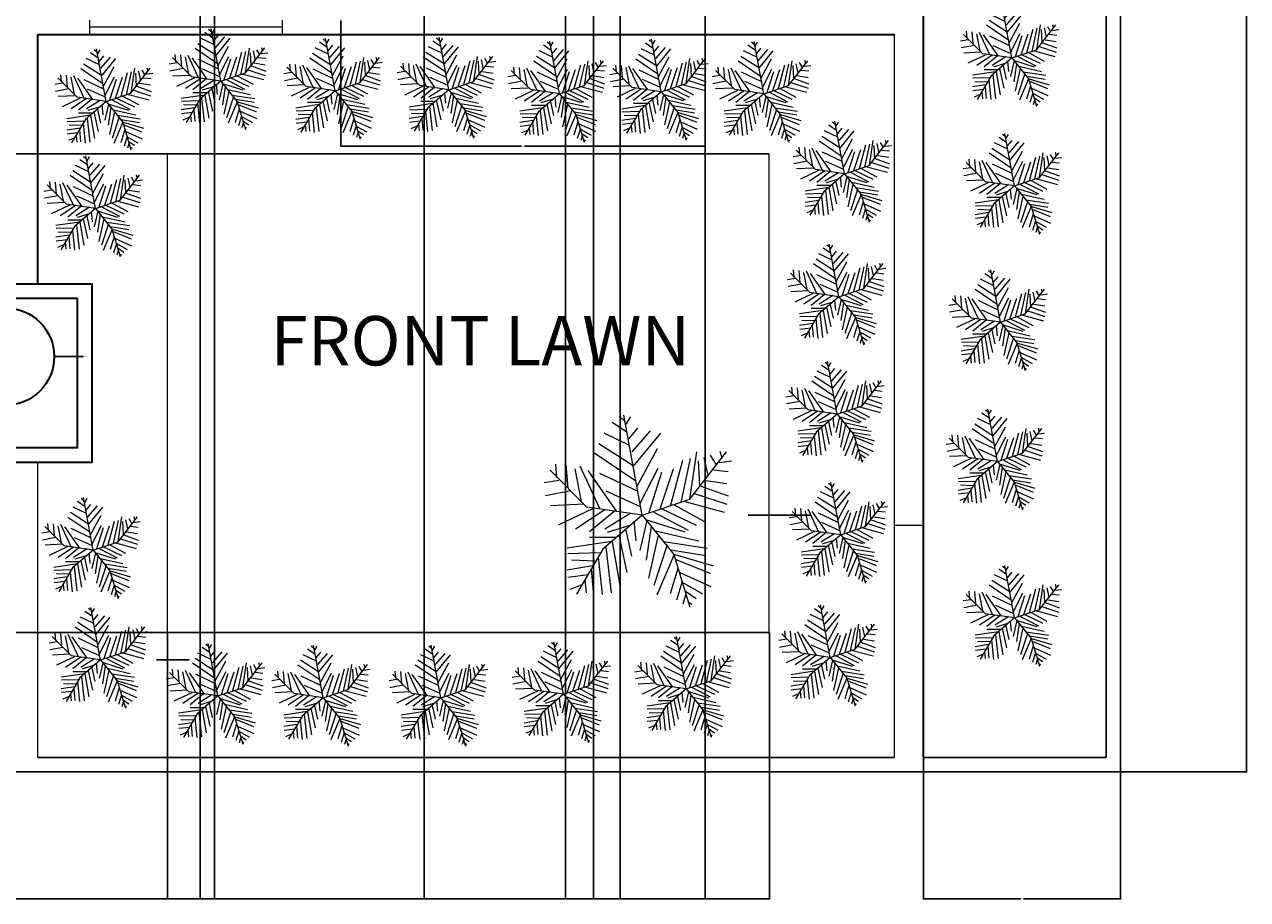
# Model space of a CAD drawing. Units: inches. Extents: x -86 to 773, y -188 to 560.
# Tile 4 of 6: x 392 to 773, y -188 to 85. Entities that reach past the tile are written whole.
import ezdxf

# ---------------------------------------------------------------- set-up
doc = ezdxf.new("R2010")
doc.units = ezdxf.units.IN
doc.header["$MEASUREMENT"] = 0
for name, color, linetype, lineweight in [('A-ANNO-DIMS', 2, 'Continuous', 18), ('A-AREA-IDEN', 7, 'Continuous', 25), ('A-COLS', 7, 'Continuous', 35), ('A-GLAZ', 7, 'Continuous', 18), ('A-WALL', 7, 'Continuous', 35), ('C-PROP', 7, 'Continuous', 25), ('L-HRDS', 7, 'Continuous', 18), ('L-PLNT', 8, 'Continuous', 13), ('L-PLNT-TREE', 8, 'Continuous', 9)]:
    doc.layers.add(name, color=color, linetype=linetype, lineweight=lineweight)
doc.styles.get("Standard").update_dxf_attribs({"font": 'arial.ttf'})
doc.dimstyles.get("Standard").update_dxf_attribs({"dimtxt": 0.18, "dimasz": 0.18, "dimexe": 0.18, "dimexo": 0.0625, "dimgap": 0.09, "dimtad": 0, "dimtih": 1, "dimtoh": 1, "dimdec": 4, "dimzin": 0, "dimdsep": 46, "dimtxsty": 'Standard', "dimcen": 0.09, "dimadec": 0, "dimazin": 0, "dimtfac": 1, "dimtdec": 4, "dimtofl": 0, "dimtmove": 0, "dimatfit": 3, "dimfxl": 1, "dimtolj": 1, "dimtzin": 0, "dimarcsym": 0})

# ---------------------------------------------------------------- blocks, each defined once
blk = doc.blocks.new('Trees - Metric')
for p, q in [((-258.7244, 1362.456), (-332.3336, 1421.4348)), ((0, 0), (-266.7, 1447.8)), ((-231.1146, 1315.2628), (-166.7002, 1421.4348)), ((-221.9198, 1197.3052), (-433.5526, 1338.8594)), ((-194.31, 1102.9442), (-65.4812, 1256.284)), ((-185.1152, 1008.5578), (-553.1612, 1185.4942)), ((-148.3106, 914.1968), (118.5418, 1220.9018)), ((-129.8956, 701.8528), (265.7602, 1185.4942)), ((-93.091, 489.5342), (-700.3796, 902.3858)), ((-129.8956, 713.6638), (-626.7704, 1032.1544)), ((-74.7014, 418.7444), (219.7608, 961.39)), ((685.8, 228.6), (1219.2, 914.4)), ((689.0258, 230.0224), (790.2448, 914.1968)), ((1121.4862, 925.9824), (1149.0706, 831.6214)), ((-1234.059, 536.7274), (-1252.4486, 737.2604)), ((-1105.2302, 725.4494), (-1077.6458, 395.1732)), ((-902.8176, 713.6638), (-617.5756, 100.2538)), ((412.9786, 147.447), (587.8068, 796.2392)), ((560.197, 182.8292), (698.2206, 819.8358)), ((808.6344, 784.4282), (827.0494, 418.7444)), ((891.4384, 831.6214), (946.658, 572.1096)), ((983.4626, 867.0036), (1066.2666, 725.4494)), ((1112.2914, 760.8316), (1296.3144, 784.4282)), ((-800.1, 114.3), (-1333.5, 647.7)), ((-976.4268, 666.4706), (-884.4026, 194.6402)), ((-369.1382, 53.086), (-783.1836, 642.874)), ((-617.5756, 607.4918), (-74.7014, 347.98)), ((-28.6766, 171.0436), (228.9556, 678.2816)), ((100.1268, 41.275), (284.1498, 619.2774)), ((256.5654, 88.4682), (449.7832, 666.4706)), ((1029.462, 654.685), (1241.0948, 631.0884)), ((-1206.4492, 501.3198), (-1418.082, 465.9376)), ((845.439, 418.7444), (1241.0948, 277.1902)), ((919.0482, 501.3198), (1222.6798, 454.152)), ((-1031.621, 347.98), (-1399.667, 277.1902)), ((-525.5514, 347.98), (-28.6766, 123.8504)), ((0, 0), (685.8, 228.6)), ((615.4166, 194.6402), (1185.8752, 41.275)), ((753.4148, 312.5978), (1222.6798, 159.2326)), ((-847.598, 159.2326), (-1326.0578, 135.636)), ((-718.7946, 88.4682), (-1215.644, -147.447)), ((-543.9664, 76.6572), (-967.2066, -206.4512)), ((0, 0), (-800.1, 114.3)), ((-405.9428, 53.086), (-764.794, -241.8334)), ((0, 0), (-571.5, -495.3)), ((-166.7002, 29.4894), (-543.9664, -206.4512)), ((0, 0), (457.2, -571.5)), ((164.5412, 41.275), (661.416, -218.2368)), ((284.1498, 88.4682), (781.0246, -147.447)), ((458.978, 147.447), (891.4384, -88.4682)), ((-166.7002, -147.447), (-507.1618, -253.619)), ((-120.7008, -88.4682), (-93.091, -371.5766)), ((63.3222, -76.6826), (-37.8714, -513.1308)), ((44.9326, -64.897), (615.4166, -241.8334)), ((127.7366, -159.258), (54.1274, -654.685)), ((-387.5278, -324.4088), (-764.794, -324.4088)), ((-341.5284, -289.0012), (-221.9198, -831.6214)), ((-240.3094, -218.2368), (-157.5054, -595.7062)), ((228.9556, -289.0012), (90.932, -914.1968)), ((192.151, -230.0224), (817.8292, -371.5766)), ((-442.7474, -383.3876), (-1086.8406, -477.7486)), ((-571.5, -495.3), (-952.5, -1143)), ((-525.5514, -465.963), (-451.9422, -1126.5408)), ((-433.5526, -383.3876), (-323.1134, -1020.3688)), ((357.759, -430.5554), (164.5412, -1020.3688)), ((311.7596, -383.3876), (937.4378, -477.7486)), ((412.9786, -501.3452), (919.0482, -583.9206)), ((-617.5756, -548.5384), (-1077.6458, -560.324)), ((-681.9646, -666.496), (-1022.4262, -654.685)), ((-635.9652, -607.5172), (-580.771, -1150.1374)), ((458.978, -572.1096), (210.5406, -1161.923)), ((457.2, -571.5), (685.8, -1333.5)), ((468.1982, -572.1096), (1029.462, -737.2604)), ((486.5878, -642.8994), (983.4626, -843.4324)), ((-718.7946, -737.2604), (-1086.8406, -796.2392)), ((-783.1836, -867.029), (-1077.6458, -902.4112)), ((-737.1842, -784.4536), (-709.5744, -1114.7298)), ((514.1976, -772.6426), (403.7838, -1138.3264)), ((541.8074, -831.6214), (992.6574, -1032.1544)), ((-875.2078, -1008.5832), (-1040.8412, -1079.3476)), ((-829.2084, -937.7934), (-810.7934, -1126.5408)), ((578.612, -961.39), (495.7826, -1232.7128)), ((578.612, -973.1756), (873.0488, -1138.3264)), ((624.6114, -1161.923), (587.8068, -1291.6916)), ((624.6114, -1102.9442), (781.0246, -1209.1162)), ((679.8056, -1268.095), (716.6102, -1291.6916))]:
    blk.add_line(p, q)
blk = doc.blocks.new('WIN-60-W4_5')
for p, q in [((0, 4.5), (0, 0)), ((60, 4.5), (60, 0)), ((60, 2.25), (0, 2.25))]:
    blk.add_line(p, q)
blk = doc.blocks.new('PORCH-COLUMN-PLINTH')
for points in [[(0, 55.74), (51.99, 55.74), (51.99, 0), (0, 0)], [(4.5, 51.24), (47.49, 51.24), (47.49, 4.5), (4.5, 4.5)]]:
    blk.add_lwpolyline(points, close=True)
blk = doc.blocks.new('*D46')
at = {"layer": 'A-ANNO-DIMS', "color": 0, "lineweight": -2, "transparency": 16777216}
for p, q in [((733.51, 486.66), (772.88, 486.66)), ((772.7, 486.48), (772.7, 169.55)), ((772.7, -147.74), (772.7, 169.19)), ((733.51, -147.92), (772.88, -147.92))]:
    blk.add_line(p, q, dxfattribs=at)
at = {"layer": 'A-ANNO-DIMS', "color": 0, "transparency": 16777216}
for points in [[(772.67, 486.48), (772.73, 486.48), (772.7, 486.66)], [(772.67, -147.74), (772.73, -147.74), (772.7, -147.92)]]:
    blk.add_solid(points, dxfattribs=at)
at = {"layer": 'Defpoints', "color": 0, "transparency": 16777216}
for p in [(733.45, 486.66), (772.7, 486.66), (733.45, -147.92)]:
    blk.add_point(p, dxfattribs=at)
at = {"layer": 'A-ANNO-DIMS', "color": 0, "transparency": 16777216, "insert": (772.7, 169.37), "char_height": 0.18, "attachment_point": 5}
blk.add_mtext('\\A1;634.6', dxfattribs=at)
blk = doc.blocks.new('*D48')
at = {"layer": 'A-ANNO-DIMS', "color": 0, "lineweight": -2, "transparency": 16777216}
for p, q in [((672.01, -143.48), (672.01, -187.76)), ((733.45, -147.98), (733.45, -187.76)), ((672.19, -187.58), (702.34, -187.58)), ((733.27, -187.58), (703.13, -187.58))]:
    blk.add_line(p, q, dxfattribs=at)
at = {"layer": 'A-ANNO-DIMS', "color": 0, "transparency": 16777216}
for points in [[(672.19, -187.55), (672.19, -187.61), (672.01, -187.58)], [(733.27, -187.55), (733.27, -187.61), (733.45, -187.58)]]:
    blk.add_solid(points, dxfattribs=at)
at = {"layer": 'Defpoints', "color": 0, "transparency": 16777216}
for p in [(672.01, -143.42), (733.45, -147.92), (733.45, -187.58)]:
    blk.add_point(p, dxfattribs=at)
at = {"layer": 'A-ANNO-DIMS', "color": 0, "transparency": 16777216, "insert": (702.73, -187.58), "char_height": 0.18, "attachment_point": 5}
blk.add_mtext('\\A1;61.44', dxfattribs=at)
blk = doc.blocks.new('*D52')
at = {"layer": 'A-ANNO-DIMS', "color": 0, "lineweight": -2, "transparency": 16777216}
for p, q in [((436.42, -104.53), (436.42, -187.76)), ((623.99, -104.5), (623.99, -187.76)), ((436.6, -187.58), (529.75, -187.58)), ((623.81, -187.58), (530.66, -187.58))]:
    blk.add_line(p, q, dxfattribs=at)
at = {"layer": 'A-ANNO-DIMS', "color": 0, "transparency": 16777216}
for points in [[(436.6, -187.55), (436.6, -187.61), (436.42, -187.58)], [(623.81, -187.55), (623.81, -187.61), (623.99, -187.58)]]:
    blk.add_solid(points, dxfattribs=at)
at = {"layer": 'Defpoints', "color": 0, "transparency": 16777216}
for p in [(436.42, -104.46), (623.99, -104.44), (623.99, -187.58)]:
    blk.add_point(p, dxfattribs=at)
at = {"layer": 'A-ANNO-DIMS', "color": 0, "transparency": 16777216, "insert": (530.2, -187.58), "char_height": 0.18, "attachment_point": 5}
blk.add_mtext('\\A1;187.57', dxfattribs=at)
blk = doc.blocks.new('*D53')
at = {"layer": 'A-ANNO-DIMS', "color": 0, "lineweight": -2, "transparency": 16777216}
for p, q in [((623.74, 44.83), (-85.98, 44.83)), ((-85.8, 44.65), (-85.8, -29.62)), ((-85.8, -104.26), (-85.8, -29.99)), ((623.93, -104.44), (-85.98, -104.44))]:
    blk.add_line(p, q, dxfattribs=at)
at = {"layer": 'A-ANNO-DIMS', "color": 0, "transparency": 16777216}
for points in [[(-85.83, 44.65), (-85.77, 44.65), (-85.8, 44.83)], [(-85.83, -104.26), (-85.77, -104.26), (-85.8, -104.44)]]:
    blk.add_solid(points, dxfattribs=at)
at = {"layer": 'Defpoints', "color": 0, "transparency": 16777216}
for p in [(623.81, 44.83), (-85.8, -104.44), (623.99, -104.44)]:
    blk.add_point(p, dxfattribs=at)
at = {"layer": 'A-ANNO-DIMS', "color": 0, "transparency": 16777216, "insert": (-85.8, -29.81), "char_height": 0.18, "attachment_point": 5}
blk.add_mtext('\\A1;149.27', dxfattribs=at)
blk = doc.blocks.new('*D54')
at = {"layer": 'A-ANNO-DIMS', "color": 0, "lineweight": -2, "transparency": 16777216}
for p, q in [((451.03, 440.67), (451.03, -187.76)), ((569.11, 440.67), (569.11, -187.76)), ((451.21, -187.58), (509.62, -187.58)), ((568.93, -187.58), (510.53, -187.58))]:
    blk.add_line(p, q, dxfattribs=at)
at = {"layer": 'A-ANNO-DIMS', "color": 0, "transparency": 16777216}
for points in [[(451.21, -187.55), (451.21, -187.61), (451.03, -187.58)], [(568.93, -187.55), (568.93, -187.61), (569.11, -187.58)]]:
    blk.add_solid(points, dxfattribs=at)
at = {"layer": 'Defpoints', "color": 0, "transparency": 16777216}
for p in [(451.03, 440.74), (569.11, 440.74), (569.11, -187.58)]:
    blk.add_point(p, dxfattribs=at)
at = {"layer": 'A-ANNO-DIMS', "color": 0, "transparency": 16777216, "insert": (510.07, -187.58), "char_height": 0.18, "attachment_point": 5}
blk.add_mtext('\\A1;118.08', dxfattribs=at)
blk = doc.blocks.new('*D65')
at = {"layer": 'A-ANNO-DIMS', "color": 0, "lineweight": -2, "transparency": 16777216}
for p, q in [((446.53, 366.45), (446.53, -187.76)), ((215.06, 361.95), (215.06, -187.76)), ((215.24, -187.58), (330.33, -187.58)), ((446.35, -187.58), (331.26, -187.58))]:
    blk.add_line(p, q, dxfattribs=at)
at = {"layer": 'A-ANNO-DIMS', "color": 0, "transparency": 16777216}
for points in [[(215.24, -187.55), (215.24, -187.61), (215.06, -187.58)], [(446.35, -187.55), (446.35, -187.61), (446.53, -187.58)]]:
    blk.add_solid(points, dxfattribs=at)
at = {"layer": 'Defpoints', "color": 0, "transparency": 16777216}
for p in [(446.53, 366.52), (215.06, 362.02), (446.53, -187.58)]:
    blk.add_point(p, dxfattribs=at)
at = {"layer": 'A-ANNO-DIMS', "color": 0, "transparency": 16777216, "insert": (330.8, -187.58), "char_height": 0.18, "attachment_point": 5}
blk.add_mtext('\\A1;231.47', dxfattribs=at)
blk = doc.blocks.new('*D71')
at = {"layer": 'A-ANNO-DIMS', "color": 0, "lineweight": -2, "transparency": 16777216}
for p, q in [((490.39, 86.43), (490.39, 47.07)), ((603.97, 86.43), (603.97, 47.07)), ((490.57, 47.25), (546.73, 47.25)), ((603.79, 47.25), (547.64, 47.25))]:
    blk.add_line(p, q, dxfattribs=at)
at = {"layer": 'A-ANNO-DIMS', "color": 0, "transparency": 16777216}
for points in [[(490.57, 47.28), (490.57, 47.22), (490.39, 47.25)], [(603.79, 47.28), (603.79, 47.22), (603.97, 47.25)]]:
    blk.add_solid(points, dxfattribs=at)
at = {"layer": 'Defpoints', "color": 0, "transparency": 16777216}
for p in [(490.39, 86.5), (603.97, 86.5), (490.39, 47.25)]:
    blk.add_point(p, dxfattribs=at)
at = {"layer": 'A-ANNO-DIMS', "color": 0, "transparency": 16777216, "insert": (547.18, 47.25), "char_height": 0.18, "attachment_point": 5}
blk.add_mtext('\\A1;113.58', dxfattribs=at)
blk = doc.blocks.new('*D72')
at = {"layer": 'A-ANNO-DIMS', "color": 0, "lineweight": -2, "transparency": 16777216}
for p, q in [((560.48, 361.95), (560.48, -187.76)), ((603.97, 361.95), (603.97, -187.76)), ((560.66, -187.58), (581.76, -187.58)), ((603.79, -187.58), (582.69, -187.58))]:
    blk.add_line(p, q, dxfattribs=at)
at = {"layer": 'A-ANNO-DIMS', "color": 0, "transparency": 16777216}
for points in [[(560.66, -187.55), (560.66, -187.61), (560.48, -187.58)], [(603.79, -187.55), (603.79, -187.61), (603.97, -187.58)]]:
    blk.add_solid(points, dxfattribs=at)
at = {"layer": 'Defpoints', "color": 0, "transparency": 16777216}
for p in [(560.48, 362.01), (603.97, 362.02), (603.97, -187.58)]:
    blk.add_point(p, dxfattribs=at)
at = {"layer": 'A-ANNO-DIMS', "color": 0, "transparency": 16777216, "insert": (582.22, -187.58), "char_height": 0.18, "attachment_point": 5}
blk.add_mtext('\\A1;43.496', dxfattribs=at)
blk = doc.blocks.new('*D74')
at = {"layer": 'A-ANNO-DIMS', "color": 0, "lineweight": -2, "transparency": 16777216}
for p, q in [((516.4, 181.21), (516.4, -187.76)), ((577.46, 181.21), (577.46, -187.76)), ((516.58, -187.58), (546.54, -187.58)), ((577.28, -187.58), (547.32, -187.58))]:
    blk.add_line(p, q, dxfattribs=at)
at = {"layer": 'A-ANNO-DIMS', "color": 0, "transparency": 16777216}
for points in [[(516.58, -187.55), (516.58, -187.61), (516.4, -187.58)], [(577.28, -187.55), (577.28, -187.61), (577.46, -187.58)]]:
    blk.add_solid(points, dxfattribs=at)
at = {"layer": 'Defpoints', "color": 0, "transparency": 16777216}
for p in [(516.4, 181.27), (577.46, 181.27), (577.46, -187.58)]:
    blk.add_point(p, dxfattribs=at)
at = {"layer": 'A-ANNO-DIMS', "color": 0, "transparency": 16777216, "insert": (546.93, -187.58), "char_height": 0.18, "attachment_point": 5}
blk.add_mtext('\\A1;61.06', dxfattribs=at)
blk = doc.blocks.new('*D89')
at = {"layer": 'A-ANNO-DIMS', "color": 0, "lineweight": -2, "transparency": 16777216}
for p, q in [((584.28, -67.83), (584.46, -67.83)), ((584.37, -67.92), (584.37, -67.74)), ((636.91, -67.83), (617.39, -67.83))]:
    blk.add_line(p, q, dxfattribs=at)
at = {"layer": 'A-ANNO-DIMS', "color": 0, "transparency": 16777216}
blk.add_solid([(617.39, -67.8), (617.39, -67.86), (617.21, -67.83)], dxfattribs=at)
at = {"layer": 'Defpoints', "color": 0, "transparency": 16777216}
for p in [(551.53, -67.83), (617.21, -67.83)]:
    blk.add_point(p, dxfattribs=at)
at = {"layer": 'A-ANNO-DIMS', "color": 0, "transparency": 16777216, "insert": (637.41, -67.83), "char_height": 0.18, "attachment_point": 5}
blk.add_mtext('\\A1;∅65.68', dxfattribs=at)
blk = doc.blocks.new('*D90')
at = {"layer": 'A-ANNO-DIMS', "color": 0, "lineweight": -2, "transparency": 16777216}
for p, q in [((415.45, -113.03), (415.63, -113.03)), ((415.54, -113.12), (415.54, -112.94)), ((443.09, -113.03), (432.94, -113.03))]:
    blk.add_line(p, q, dxfattribs=at)
at = {"layer": 'A-ANNO-DIMS', "color": 0, "transparency": 16777216}
blk.add_solid([(432.94, -113), (432.94, -113.06), (432.76, -113.03)], dxfattribs=at)
at = {"layer": 'Defpoints', "color": 0, "transparency": 16777216}
for p in [(398.32, -113.03), (432.76, -113.03)]:
    blk.add_point(p, dxfattribs=at)
at = {"layer": 'A-ANNO-DIMS', "color": 0, "transparency": 16777216, "insert": (443.84, -113.03), "char_height": 0.18, "attachment_point": 5}
blk.add_mtext('\\A1;47X ∅34.44', dxfattribs=at)
blk = doc.blocks.new('*D92')
at = {"layer": 'A-ANNO-DIMS', "color": 0, "lineweight": -2, "transparency": 16777216}
for p, q in [((385.79, -18.42), (385.97, -18.42)), ((385.88, -18.51), (385.88, -18.33)), ((410.18, -18.42), (401.25, -18.42))]:
    blk.add_line(p, q, dxfattribs=at)
at = {"layer": 'A-ANNO-DIMS', "color": 0, "transparency": 16777216}
blk.add_solid([(401.25, -18.39), (401.25, -18.45), (401.07, -18.42)], dxfattribs=at)
at = {"layer": 'Defpoints', "color": 0, "transparency": 16777216}
for p in [(370.7, -18.42), (401.07, -18.42)]:
    blk.add_point(p, dxfattribs=at)
at = {"layer": 'A-ANNO-DIMS', "color": 0, "transparency": 16777216, "insert": (410.67, -18.42), "char_height": 0.18, "attachment_point": 5}
blk.add_mtext('\\A1;∅30.37', dxfattribs=at)

msp = doc.modelspace()

# ---------------------------------------------------------------- linework, layer by layer
at = {"layer": 'A-COLS'}
msp.add_circle((385.883, -18.4243), 15.1853, dxfattribs=at)
at = {"layer": 'A-WALL'}
for p, q in [((672.0115, -143.4172), (672.0115, 366.5167)), ((395.9662, 4.3272), (395.9662, 81.9967))]:
    msp.add_line(p, q, dxfattribs=at)
msp.add_lwpolyline([(395.9662, 81.9967), (663.0115, 81.9967)], dxfattribs=at)
at = {"layer": 'C-PROP'}
for p, q in [((733.4515, -147.9172), (733.4515, 486.6589)), ((728.9515, -143.4172), (728.9515, 482.1589)), ((395.9662, -143.4172), (663.0115, -143.4172)), ((672.0115, -143.4172), (728.9515, -143.4172)), ((269.2915, -147.9172), (733.4515, -147.9172))]:
    msp.add_line(p, q, dxfattribs=at)
at = {"layer": 'L-HRDS'}
for p, q in [((663.0115, -143.4172), (663.0115, 81.9967)), ((395.9662, -143.4172), (395.9662, -51.4118))]:
    msp.add_line(p, q, dxfattribs=at)
msp.add_lwpolyline([(663.0115, -70.9433), (672.0115, -70.9433)], dxfattribs=at)
at = {"layer": 'L-PLNT'}
msp.add_lwpolyline([(436.4196, 44.8288), (623.8051, 44.8288), (623.8051, -104.464), (436.4196, -104.464)], close=True, dxfattribs=at)

# ---------------------------------------------------------------- block references
at = {"layer": 'A-COLS'}
msp.add_blockref('PORCH-COLUMN-PLINTH', (360.7615, -51.4123), dxfattribs=at)
at = {"layer": 'A-GLAZ'}
msp.add_blockref('WIN-60-W4_5', (412.1017, 82.0297), dxfattribs=at)
at = {"layer": 'L-PLNT-TREE'}
for p, xscale, yscale, zscale in [((699.5311, 74.7194), 0.0112992005060107, 0.0112992005060107, 0.0112992005060107), ((452.9609, 67.5005), 0.0112992005060107, 0.0112992005060107, 0.0112992005060107), ((488.6741, 64.4994), 0.0112992005060107, 0.0112992005060107, 0.0112992005060107), ((524.0319, 64.8152), 0.0112992005060107, 0.0112992005060107, 0.0112992005060107), ((590.2526, 64.1811), 0.0112992005060107, 0.0112992005060107, 0.0112992005060107), ((417.2477, 61.1649), 0.0112992005060107, 0.0112992005060107, 0.0112992005060107), ((558.5174, 63.547), 0.0112992005060107, 0.0112992005060107, 0.0112992005060107), ((622.1993, 63.547), 0.0112992005060107, 0.0112992005060107, 0.0112992005060107), ((647.3758, 38.6056), 0.0112992005060107, 0.0112992005060107, 0.0112992005060107), ((700.4182, 34.8337), 0.0112992005060107, 0.0112992005060107, 0.0112992005060107), ((413.91, 27.8195), 0.0112992005060107, 0.0112992005060107, 0.0112992005060107), ((645.6489, 0.2733), 0.0112992005060107, 0.0112992005060107, 0.0112992005060107), ((695.9823, -7.7111), 0.0112992005060107, 0.0112992005060107, 0.0112992005060107), ((645.1021, -36.3229), 0.0112992005060107, 0.0112992005060107, 0.0112992005060107), ((584.3675, -67.8322), 0.0215496520476157, 0.0215496520476157, 0.0215496520476157), ((695.0951, -51.1423), 0.0112992005060107, 0.0112992005060107, 0.0112992005060107), ((646.1956, -74.0115), 0.0112992005060107, 0.0112992005060107, 0.0112992005060107), ((413.2487, -78.7518), 0.0112992005060107, 0.0112992005060107, 0.0112992005060107), ((700.4182, -99.8916), 0.0112992005060107, 0.0112992005060107, 0.0112992005060107), ((415.5387, -113.0331), 0.0112992005060107, 0.0112992005060107, 0.0112992005060107), ((642.9152, -112.2464), 0.0112992005060107, 0.0112992005060107, 0.0112992005060107), ((598.0835, -122.0782), 0.0112992005060107, 0.0112992005060107, 0.0112992005060107), ((452.1069, -124.263), 0.0112992005060107, 0.0112992005060107, 0.0112992005060107), ((484.9106, -124.8093), 0.0112992005060107, 0.0112992005060107, 0.0112992005060107), ((521.5414, -124.8093), 0.0112992005060107, 0.0112992005060107, 0.0112992005060107), ((559.8125, -123.7168), 0.0112992005060107, 0.0112992005060107, 0.0112992005060107)]:
    msp.add_blockref('Trees - Metric', p, dxfattribs=dict(at, xscale=xscale, yscale=yscale, zscale=zscale))

# ---------------------------------------------------------------- texts
at = {"layer": 'A-AREA-IDEN'}
msp.add_text('FRONT LAWN', height=15.3913, dxfattribs=at).set_placement((468.5175, -21.1684))

# ---------------------------------------------------------------- dimensions: what is measured, and where the dimension line sits
at = {"layer": 'A-ANNO-DIMS'}
for base, p1, p2, angle, override, picture, middle in [((772.7015, 486.6589), (733.4515, -147.9172), (733.4515, 486.6589), 90, {"dimdec": 1, "dimlfac": 1, "dimrnd": 0, "dimzin": 0, "dimdsep": 46, "dimlunit": 2}, '*D46', (772.7015, 169.3709)), ((490.3915, 47.2467), (603.9715, 86.4967), (490.3915, 86.4967), 180, {"dimdec": 2, "dimlfac": 1, "dimrnd": 0, "dimzin": 0, "dimdsep": 46, "dimlunit": 2}, '*D71', (547.1815, 47.2467)), ((-85.7985, -104.4394), (623.8051, 44.8288), (623.9902, -104.4394), 90, {"dimdec": 2, "dimlfac": 1, "dimrnd": 0, "dimzin": 0, "dimdsep": 46, "dimlunit": 2}, '*D53', (-85.7985, -29.8053))]:
    dim = msp.add_linear_dim(base=base, p1=p1, p2=p2, angle=angle, dimstyle='Standard', override=override, dxfattribs=at)
    dim.commit()
    dim.dimension.update_dxf_attribs({"geometry": picture, "text_midpoint": middle})
for base, p1, p2, override, picture, middle in [((569.1115, -187.578), (451.0315, 440.7367), (569.1115, 440.7367), {"dimdec": 2, "dimlfac": 1, "dimrnd": 0, "dimzin": 0, "dimdsep": 46, "dimlunit": 2}, '*D54', (510.0715, -187.578)), ((446.5315, -187.578), (215.0615, 362.0167), (446.5315, 366.5167), {"dimdec": 2, "dimlfac": 1, "dimrnd": 0, "dimzin": 0, "dimdsep": 46, "dimlunit": 2}, '*D65', (330.7965, -187.578)), ((603.9715, -187.578), (560.4759, 362.0116), (603.9715, 362.0167), {"dimdec": 3, "dimlfac": 1, "dimrnd": 0, "dimzin": 0, "dimdsep": 46, "dimlunit": 2}, '*D72', (582.2237, -187.578)), ((577.46, -187.578), (516.4009, 181.2736), (577.46, 181.2736), {"dimdec": 2, "dimlfac": 1, "dimrnd": 0, "dimzin": 0, "dimdsep": 46, "dimlunit": 2}, '*D74', (546.9304, -187.578)), ((623.9902, -187.578), (436.4196, -104.464), (623.9902, -104.4394), {"dimdec": 2, "dimlfac": 1, "dimrnd": 0, "dimzin": 0, "dimdsep": 46, "dimlunit": 2}, '*D52', (530.2049, -187.578)), ((733.4515, -187.578), (672.0115, -143.4172), (733.4515, -147.9172), {"dimdec": 2, "dimlfac": 1, "dimrnd": 0, "dimzin": 0, "dimdsep": 46, "dimlunit": 2}, '*D48', (702.7315, -187.578))]:
    dim = msp.add_linear_dim(base=base, p1=p1, p2=p2, dimstyle='Standard', override=override, dxfattribs=at)
    dim.commit()
    dim.dimension.update_dxf_attribs({"geometry": picture, "text_midpoint": middle})
for p1, p2, picture, middle in [((370.6977, -18.4245), (401.0683, -18.424), '*D92', (410.1794, -18.4238)), ((551.5258, -67.8324), (617.2092, -67.832), '*D89', (636.9142, -67.8319))]:
    dim = msp.add_diameter_dim_2p(p1=p1, p2=p2, dimstyle='Standard', override={"dimdec": 2, "dimlfac": 1, "dimrnd": 0, "dimzin": 0, "dimdsep": 46, "dimlunit": 2}, dxfattribs=at)
    dim.commit()
    dim.dimension.update_dxf_attribs({"geometry": picture, "text_midpoint": middle, "dimtype": 163})
dim = msp.add_diameter_dim_2p(p1=(398.3187, -113.0332), p2=(432.7587, -113.033), text='47X <>', dimstyle='Standard', override={"dimdec": 2, "dimlfac": 1, "dimrnd": 0, "dimzin": 0, "dimdsep": 46, "dimlunit": 2}, dxfattribs=at)
dim.commit()
dim.dimension.update_dxf_attribs({"geometry": '*D90', "text_midpoint": (443.0907, -113.0329), "dimtype": 163})

doc.saveas('drawing.dxf')
